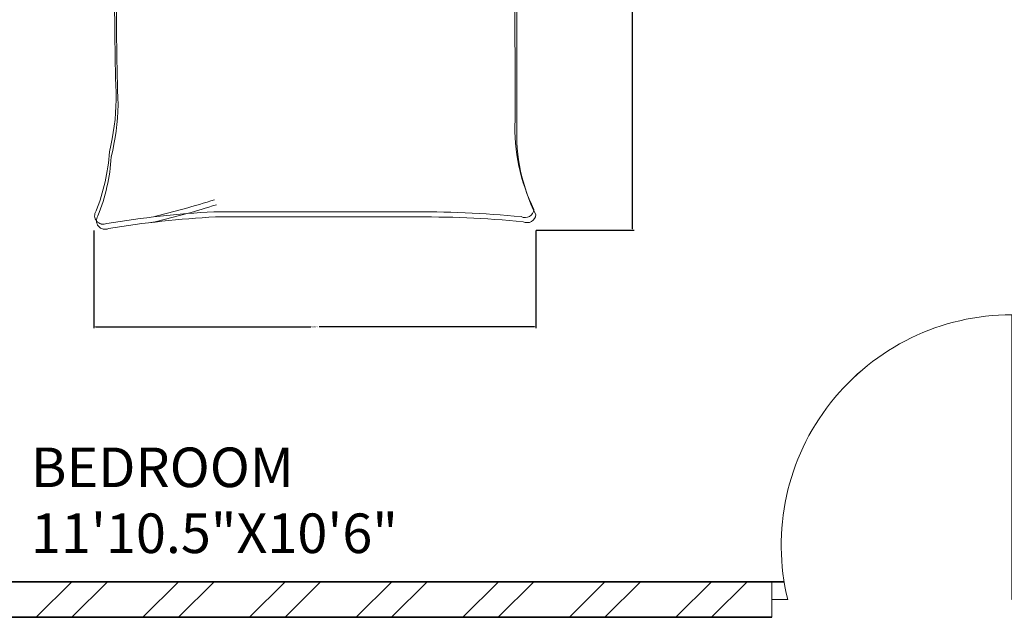
# Model space of a CAD drawing. Units: inches. Extents: x 2120 to 4013, y 1390 to 3019.
# Tile 40 of 59: x 2736 to 2861, y 2213 to 2289. Entities that reach past the tile are written whole.
import ezdxf

# ---------------------------------------------------------------- set-up
doc = ezdxf.new("R2010")
doc.units = ezdxf.units.IN
for name, color, linetype, lineweight in [('A-ANNO-DIMS', 2, 'Continuous', 18), ('A-AREA-IDEN', 7, 'Continuous', 18), ('A-DOOR', 3, 'Continuous', 18), ('A-FURN', 8, 'Continuous', 13), ('A-WALL', 7, 'Continuous', 35), ('A-WALL-PATT', 252, 'Continuous', 13)]:
    doc.layers.add(name, color=color, linetype=linetype, lineweight=lineweight)
doc.styles.get("Standard").update_dxf_attribs({"font": 'arial.ttf'})
doc.dimstyles.get("Standard").update_dxf_attribs({"dimtxt": 0.18, "dimasz": 0.18, "dimexe": 0.18, "dimexo": 0.0625, "dimgap": 0.09, "dimtad": 0, "dimtih": 1, "dimtoh": 1, "dimdec": 4, "dimzin": 0, "dimdsep": 46, "dimtxsty": 'Standard', "dimcen": 0.09, "dimadec": 0, "dimazin": 0, "dimtfac": 1, "dimtdec": 4, "dimtofl": 0, "dimtmove": 0, "dimatfit": 3, "dimfxl": 1, "dimtolj": 1, "dimtzin": 0, "dimarcsym": 0})

# ---------------------------------------------------------------- blocks, each defined once
blk = doc.blocks.new('BED-DOUBLE-PLAN')
for p, q in [((3.48, 63.34), (3.48, 81.45)), ((3.48, 81.45), (51.27, 81.45)), ((51.27, 81.45), (51.27, 54.84)), ((3.48, 79.91), (51.27, 79.91)), ((3.7, 62.7), (3.7, 80.81)), ((51.5, 80.81), (51.5, 54.2)), ((3.7, 79.27), (51.5, 79.27)), ((3.9, 78.11), (8.18, 78.44)), ((8.18, 78.44), (8.29, 78.42)), ((8.29, 78.42), (12.11, 78.13)), ((14.86, 77.7), (16.88, 78.42)), ((16.88, 78.42), (19.77, 79.14)), ((17.11, 77.78), (20, 78.5)), ((19.77, 79.14), (20.09, 79.14)), ((20, 78.5), (20.32, 78.5)), ((20.09, 79.14), (24.54, 79)), ((20.32, 78.5), (24.77, 78.36)), ((24.54, 79), (25.98, 79.58)), ((24.77, 78.36), (26.21, 78.94)), ((25.98, 79.58), (26.56, 74.23)), ((26.21, 78.94), (26.79, 73.59)), ((27.98, 78.95), (27.73, 73.58)), ((29.46, 78.47), (27.98, 78.95)), ((33.89, 78.89), (29.46, 78.47)), ((34.21, 78.91), (33.89, 78.89)), ((37.14, 78.37), (34.21, 78.91)), ((41.92, 78.38), (36.5, 77.02)), ((45.71, 78.9), (41.92, 78.38)), ((50.11, 78.89), (44.71, 78.99)), ((44.71, 78.99), (45.71, 78.9)), ((50.11, 78.89), (49.73, 75.68)), ((3.9, 78.13), (4.47, 74.95)), ((4.12, 77.49), (4.7, 74.31)), ((4.13, 77.47), (8.41, 77.8)), ((8.41, 77.8), (8.51, 77.78)), ((8.51, 77.78), (12.34, 77.49)), ((12.11, 78.13), (17.6, 77.12)), ((12.34, 77.49), (17.83, 76.48)), ((15.08, 77.06), (17.11, 77.78)), ((28.21, 78.32), (27.96, 72.94)), ((29.69, 77.83), (28.21, 78.32)), ((34.11, 78.25), (29.69, 77.83)), ((34.43, 78.27), (34.11, 78.25)), ((37.37, 77.73), (34.43, 78.27)), ((42.14, 77.74), (36.72, 76.38)), ((39.2, 77.77), (37.14, 78.37)), ((39.43, 77.13), (37.37, 77.73)), ((45.94, 78.26), (42.14, 77.74)), ((50.34, 78.25), (44.94, 78.35)), ((44.94, 78.35), (45.94, 78.26)), ((50.34, 78.25), (49.96, 75.04)), ((4.47, 74.95), (4.04, 72.35)), ((5.05, 72.49), (6.06, 75.24)), ((49.31, 73.19), (48.13, 75.87)), ((49.54, 72.55), (48.36, 75.23)), ((49.73, 75.68), (50.33, 73.11)), ((49.96, 75.04), (50.56, 72.47)), ((4.7, 74.31), (4.27, 71.71)), ((5.28, 71.85), (6.29, 74.6)), ((26.56, 74.23), (27.14, 71.05)), ((26.79, 73.59), (27.37, 70.41)), ((27.73, 73.58), (27.36, 70.37)), ((4.04, 72.35), (4.62, 71.33)), ((4.47, 68.88), (5.05, 72.49)), ((27.96, 72.94), (27.58, 69.73)), ((50.11, 69.62), (49.31, 73.19)), ((50.34, 68.98), (49.54, 72.55)), ((50.33, 73.11), (49.82, 72.06)), ((50.56, 72.47), (50.04, 71.42)), ((4.27, 71.71), (4.85, 70.7)), ((4.7, 68.24), (5.28, 71.85)), ((27.14, 71.05), (27.14, 69.74)), ((27.14, 69.74), (26.56, 67.86)), ((27.36, 70.37), (27.44, 69.07)), ((27.37, 70.41), (27.37, 69.1)), ((27.58, 69.73), (27.67, 68.43)), ((4.76, 67.29), (4.47, 68.88)), ((27.37, 69.1), (26.79, 67.23)), ((27.44, 69.07), (28.13, 67.23)), ((27.67, 68.43), (28.36, 66.59)), ((49.92, 68.01), (50.11, 69.62)), ((50.15, 67.37), (50.34, 68.98)), ((4.19, 64.11), (4.76, 67.29)), ((4.99, 66.65), (4.7, 68.24)), ((26.56, 67.86), (26.56, 65.18)), ((26.79, 67.23), (26.79, 64.54)), ((28.13, 67.23), (28.3, 64.55)), ((50.7, 64.87), (49.92, 68.01)), ((50.93, 64.23), (50.15, 67.37)), ((4.41, 63.47), (4.99, 66.65)), ((24.1, 65.18), (20.96, 66.27)), ((28.36, 66.59), (28.53, 63.91)), ((30.75, 64.71), (33.82, 65.99)), ((9.28, 64.83), (4.19, 64.11)), ((6.38, 65.82), (10.42, 65.15)), ((6.61, 65.18), (10.64, 64.51)), ((10.42, 65.15), (9.28, 64.83)), ((10.42, 65.15), (17.43, 64.72)), ((17.43, 64.72), (19.39, 65.28)), ((19.39, 65.28), (24.52, 64.87)), ((24.33, 64.54), (21.19, 65.63)), ((26.56, 65.18), (24.1, 65.18)), ((28.3, 64.55), (30.75, 64.71)), ((30.98, 64.07), (34.05, 65.35)), ((32.57, 65.82), (36.6, 65.15)), ((32.79, 65.18), (36.83, 64.51)), ((36.6, 65.15), (43.61, 64.72)), ((43.61, 64.72), (45.57, 65.28)), ((45.57, 65.28), (50.7, 64.87)), ((9.51, 64.19), (4.41, 63.47)), ((10.64, 64.51), (9.51, 64.19)), ((10.64, 64.51), (17.65, 64.08)), ((17.65, 64.08), (19.61, 64.64)), ((19.61, 64.64), (24.75, 64.23)), ((26.79, 64.54), (24.33, 64.54)), ((28.53, 63.91), (30.98, 64.07)), ((30.26, 64.06), (34.45, 57.57)), ((40.65, 61.13), (32.31, 64.06)), ((36.83, 64.51), (43.84, 64.08)), ((43.84, 64.08), (45.8, 64.64)), ((45.8, 64.64), (50.93, 64.23)), ((30.49, 63.42), (34.68, 56.93)), ((40.87, 60.49), (32.54, 63.42)), ((46.22, 59.12), (40.65, 61.13)), ((46.45, 58.48), (40.87, 60.49)), ((49.16, 56.95), (46.22, 59.12)), ((49.39, 56.31), (46.45, 58.48)), ((34.45, 57.57), (36.15, 53.08)), ((34.68, 56.93), (36.38, 52.44)), ((52.87, 53.7), (49.16, 56.95)), ((53.1, 53.06), (49.39, 56.31)), ((51.33, 53.08), (52.87, 53.7)), ((52.95, 51.96), (52.87, 53.7, 3.87)), ((36.15, 53.08), (36.46, 51.07)), ((36.38, 52.44), (36.69, 50.43)), ((38.94, 51.69), (40.96, 52.62)), ((40.96, 52.62), (44.36, 53.08)), ((41.18, 51.98), (44.59, 52.44)), ((44.36, 53.08), (48.23, 53.39)), ((44.59, 52.44), (48.46, 52.75)), ((48.23, 53.39), (51.33, 53.08)), ((48.46, 52.75), (51.56, 52.44)), ((51.56, 52.44), (53.1, 53.06)), ((53.18, 51.32), (53.1, 53.06, 3.87)), ((36.46, 51.07), (38.94, 51.69)), ((36.69, 50.43), (39.17, 51.05)), ((39.17, 51.05), (41.18, 51.98)), ((15.06, 2.2), (39.68, 2.2)), ((15.29, 1.56), (39.91, 1.56))]:
    blk.add_line(p, q)
for centre, radius, start, end in [((21.36, -100.61), 164.97, 86.0865, 96.7821), ((21.59, -101.25), 164.97, 86.0865, 96.7821), ((85.16, 61.35), 83.31, 178.7218, 185.604), ((85.39, 60.71), 83.31, 178.7218, 185.604), ((17.76, -74.87), 129.02, 81.7845, 96.9006), ((17.99, -75.51), 129.02, 81.7845, 96.9006), ((-167.31, 50.27), 170.11, 358.4762, 1.0082), ((-167.08, 49.63), 170.11, 358.4762, 1.0082), ((43.74, 46.38), 6.22, 78.6608, 113.7384), ((51.33, 88.1), 36.18, 259.8763, 272.5657), ((36.64, 51.01), 0.185, 160.2464, 271.1377), ((31.16, 79.96), 29.65, 280.6617, 289.8806), ((31.38, 79.32), 29.65, 280.6617, 289.8806), ((43.97, 45.74), 6.22, 78.6608, 113.7384), ((51.56, 87.46), 36.18, 259.8763, 272.5657), ((182.27, 45.13), 129.5, 176.9791, 183.8365), ((182.5, 44.49), 129.5, 176.9791, 183.8365), ((36.87, 50.37), 0.185, 160.2464, 271.1377), ((484.82, 30.83), 482.31, 178.2277, 181.7185), ((485.05, 30.19), 482.31, 178.2277, 181.7185), ((-4508.74, 13.62), 4561.86, 0.00217, 0.28689), ((-4508.51, 12.99), 4561.86, 0.00217, 0.28689), ((-26.9, 16.93), 29.63, 346.0648, 358.9113), ((-26.67, 16.29), 29.63, 346.0648, 358.9113), ((76.16, 12.78), 23.07, 177.4714, 206.4681), ((76.39, 12.14), 23.07, 177.4714, 206.4681), ((-21.66, 11.17), 23.56, 337.9751, 356.652), ((-21.43, 10.53), 23.56, 337.9751, 356.652), ((-17.22, 105.16), 106.46, 283.3832, 287.7053), ((-16.99, 104.52), 106.46, 283.3832, 287.7053), ((54.41, 2.58), 1.1, 242.6588, 356.02), ((1.09, 1.73), 1.09, 146.1736, 293.4781), ((1.32, 1.09), 1.09, 146.1736, 293.4781), ((21.43, -119.39), 121.76, 92.9958, 99.4091), ((21.66, -120.03), 121.76, 92.9958, 99.4091), ((41.15, -130.83), 133.04, 84.4998, 90.6351), ((41.38, -131.47), 133.04, 84.4998, 90.6351), ((54.64, 1.94), 1.1, 242.6588, 356.02)]:
    blk.add_arc(centre, radius, start, end)
blk = doc.blocks.new('DOOR-SWING-36IN-103p63DEG')
for p, q in [((30.32, 2.25), (30.32, 38.25)), ((0, 4.5), (0, 0)), ((32.32, 4.5), (32.32, 0)), ((0, 0), (0, 2.25)), ((0, 2.25), (2, 2.25)), ((32.32, 2.25), (30.32, 2.25)), ((32.32, 0), (32.32, 2.25))]:
    blk.add_line(p, q)
blk.add_arc((30.32, 9.11), 29.14, 90, 193.6269)
blk = doc.blocks.new('*D73')
at = {"layer": 'A-ANNO-DIMS', "color": 0, "lineweight": -2, "transparency": 16777216}
for p, q in [((2801.55, 2343.53), (2813.9, 2343.53)), ((2813.72, 2343.35), (2813.72, 2302.94)), ((2813.72, 2262.16), (2813.72, 2302.57)), ((2801.55, 2261.98), (2813.9, 2261.98))]:
    blk.add_line(p, q, dxfattribs=at)
at = {"layer": 'A-ANNO-DIMS', "color": 0, "transparency": 16777216}
for points in [[(2813.69, 2343.35), (2813.75, 2343.35), (2813.72, 2343.53)], [(2813.69, 2262.16), (2813.75, 2262.16), (2813.72, 2261.98)]]:
    blk.add_solid(points, dxfattribs=at)
at = {"layer": 'Defpoints', "color": 0, "transparency": 16777216}
for p in [(2801.49, 2343.53), (2813.72, 2343.53), (2801.49, 2261.98)]:
    blk.add_point(p, dxfattribs=at)
at = {"layer": 'A-ANNO-DIMS', "color": 0, "transparency": 16777216, "insert": (2813.72, 2302.76), "char_height": 0.18, "attachment_point": 5}
blk.add_mtext('\\A1;BED 82 TYP.', dxfattribs=at)
blk = doc.blocks.new('*D74')
at = {"layer": 'A-ANNO-DIMS', "color": 0, "lineweight": -2, "transparency": 16777216}
for p, q in [((2745.67, 2261.92), (2745.67, 2249.57)), ((2801.49, 2261.92), (2801.49, 2249.57)), ((2745.85, 2249.75), (2773.05, 2249.75)), ((2801.31, 2249.75), (2774.11, 2249.75))]:
    blk.add_line(p, q, dxfattribs=at)
at = {"layer": 'A-ANNO-DIMS', "color": 0, "transparency": 16777216}
for points in [[(2745.85, 2249.78), (2745.85, 2249.72), (2745.67, 2249.75)], [(2801.31, 2249.78), (2801.31, 2249.72), (2801.49, 2249.75)]]:
    blk.add_solid(points, dxfattribs=at)
at = {"layer": 'Defpoints', "color": 0, "transparency": 16777216}
for p in [(2745.67, 2261.98), (2801.49, 2261.98), (2801.49, 2249.75)]:
    blk.add_point(p, dxfattribs=at)
at = {"layer": 'A-ANNO-DIMS', "color": 0, "transparency": 16777216, "insert": (2773.58, 2249.75), "char_height": 0.18, "attachment_point": 5}
blk.add_mtext('\\A1;56 TYP.', dxfattribs=at)

msp = doc.modelspace()

# ---------------------------------------------------------------- hatches: boundary and pattern name
at = {"layer": 'A-WALL-PATT'}
h = msp.add_hatch(dxfattribs=at)
h.set_pattern_fill('ANSI32', color=256)
h.paths.add_polyline_path([(2271.7331, 2343.531), (2283.3788, 2343.531), (2283.3788, 2348.031), (2283.3788, 2352.5306), (2262.7331, 2352.5306), (2262.7331, 2182.638), (2267.2331, 2182.638), (2271.7331, 2182.638), (2271.7331, 2219.031), (2391.7331, 2219.031), (2391.7331, 2214.189), (2393.9831, 2214.189), (2396.2331, 2214.189), (2396.2331, 2219.031), (2420.2331, 2219.031), (2420.2331, 2225.7535), (2417.2197, 2225.7535), (2415.7331, 2225.7535), (2415.7331, 2223.5306), (2271.7331, 2223.5306)])
h.paths.add_polyline_path([(2380.0942, 2352.5306), (2343.3788, 2352.5306), (2343.3788, 2343.531), (2363.2331, 2343.531), (2363.2331, 2288.8489), (2365.4831, 2288.8489), (2367.7331, 2288.8489), (2367.7331, 2343.531), (2380.0942, 2343.531)], flags=17)
h.paths.add_polyline_path([(2432.4339, 2352.5306), (2404.0943, 2352.5306), (2404.0943, 2343.531), (2415.7331, 2343.531), (2415.7331, 2264.0306), (2367.7331, 2264.0306), (2367.7331, 2266.4872), (2363.2331, 2266.4872), (2363.2331, 2259.531), (2367.7331, 2259.531), (2415.7331, 2259.531), (2415.7331, 2255.0658), (2420.2331, 2255.0658), (2420.2331, 2259.531), (2424.5717, 2259.531), (2424.5717, 2261.781), (2424.5717, 2264.0306), (2420.2331, 2264.0306), (2420.2331, 2343.531), (2432.4339, 2343.531)])
h.paths.add_polyline_path([(2508.9115, 2352.5306), (2456.4339, 2352.5306), (2456.4339, 2343.531), (2468.2331, 2343.531), (2468.2331, 2264.0306), (2448.0487, 2264.0306), (2448.0487, 2259.531), (2468.2331, 2259.531), (2468.2331, 2255.5496), (2472.7331, 2255.5496), (2472.7331, 2343.531), (2508.9115, 2343.531)])
h.paths.add_polyline_path([(2637.7331, 2352.5306), (2544.9116, 2352.5306), (2544.9116, 2343.531), (2589.7331, 2343.531), (2633.2331, 2343.531), (2637.7331, 2343.531)])
h.paths.add_polyline_path([(2594.2331, 2343.5306), (2589.7331, 2343.5306), (2589.7331, 2259.5306), (2589.7331, 2252.4915), (2591.9831, 2252.4915), (2594.2331, 2252.4915)])
h.paths.add_polyline_path([(2637.7331, 2223.5306), (2594.2331, 2223.5306), (2594.2331, 2230.1988), (2591.9831, 2230.1988), (2589.7331, 2230.1988), (2589.7331, 2223.5306), (2472.7331, 2223.5306), (2468.2331, 2223.5306), (2468.2331, 2219.031), (2628.7331, 2219.031), (2628.7331, 2138.031), (2637.7331, 2138.031)])
h.paths.add_polyline_path([(3822.6535, 2458.4402), (3874.9468, 2458.4402), (3874.9468, 2476.9866), (3822.6535, 2476.9866)], flags=9)
h.paths.add_polyline_path([(3834.6921, 2781.8174), (3935.9206, 2781.8174), (3935.9206, 2800.3638), (3834.6921, 2800.3638)], flags=9)
h.paths.add_polyline_path([(3832.2843, 2837.9683), (3884.5776, 2837.9683), (3884.5776, 2856.5146), (3832.2843, 2856.5146)], flags=9)
h.paths.add_polyline_path([(3830.9388, 2861.4782), (3956.8958, 2861.4782), (3956.8958, 2880.0245), (3830.9388, 2880.0245)], flags=9)
h.paths.add_polyline_path([(3870.6966, 2352.5752), (3887.9272, 2352.5752), (3887.9272, 2377.3037), (3870.6966, 2377.3037)], flags=9)
h.paths.add_polyline_path([(3289.2701, 2413.161), (3435.2223, 2413.161), (3435.2223, 2450.2538), (3289.2701, 2450.2538)], flags=9)
h.paths.add_polyline_path([(2487.6944, 2414.3601), (2637.8335, 2414.3601), (2637.8335, 2451.4528), (2487.6944, 2451.4528)], flags=9)
h.paths.add_polyline_path([(2567.3724, 1457.9199), (2815.296, 1457.9199), (2815.296, 1495.0127), (2567.3724, 1495.0127)], flags=9)
h.paths.add_polyline_path([(2655.3825, 2093.2363), (2685.9555, 2093.2363), (2685.9555, 2111.8937), (2655.3825, 2111.8937)], flags=9)
h.paths.add_polyline_path([(2543.9218, 1550.6671), (2587.8406, 1550.6671), (2587.8406, 1569.3244), (2543.9218, 1569.3244)], flags=9)
h.paths.add_polyline_path([(2905.1384, 1543.8113), (2949.0572, 1543.8113), (2949.0572, 1562.4686), (2905.1384, 1562.4686)], flags=9)
h.paths.add_polyline_path([(2736.4118, 1702.4736), (2784.2153, 1702.4736), (2784.2153, 1721.1309), (2736.4118, 1721.1309)], flags=9)
h.paths.add_polyline_path([(2912.8666, 1710.4168), (2951.707, 1710.4168), (2951.707, 1729.0741), (2912.8666, 1729.0741)], flags=9)
h.paths.add_polyline_path([(2923.5785, 1763.5038), (2959.7279, 1763.5038), (2959.7279, 1782.1611), (2923.5785, 1782.1611)], flags=9)
h.paths.add_polyline_path([(2925.2114, 1809.6137), (2967.1861, 1809.6137), (2967.1861, 1828.271), (2925.2114, 1828.271)], flags=9)
h.paths.add_polyline_path([(2996.2711, 1878.9003), (2996.2711, 1913.109), (2977.6138, 1913.109), (2977.6138, 1878.9003)], flags=9)
h.paths.add_polyline_path([(2883.0859, 1895.7192), (2927.1855, 1895.7192), (2927.1855, 1914.3766), (2883.0859, 1914.3766)], flags=9)
h.paths.add_polyline_path([(2787.3924, 1810.8013), (2841.0213, 1810.8013), (2841.0213, 1829.4587), (2787.3924, 1829.4587)], flags=9)
h.paths.add_polyline_path([(2775.6399, 2101.7395), (2829.2689, 2101.7395), (2829.2689, 2120.3968), (2775.6399, 2120.3968)], flags=9)
h.paths.add_polyline_path([(2913.0263, 2075.817), (2951.8667, 2075.817), (2951.8667, 2094.4744), (2913.0263, 2094.4744)], flags=9)
h.paths.add_polyline_path([(2929.966, 2133.3669), (2966.1154, 2133.3669), (2966.1154, 2152.0243), (2929.966, 2152.0243)], flags=9)
h.paths.add_polyline_path([(2932.7502, 2182.6088), (2968.8996, 2182.6088), (2968.8996, 2201.2662), (2932.7502, 2201.2662)], flags=9)
h.paths.add_polyline_path([(2996.0681, 2266.3173), (2996.0681, 2300.5261), (2977.4108, 2300.5261), (2977.4108, 2266.3173)], flags=9)
h.paths.add_polyline_path([(2885.1039, 2279.2186), (2929.2035, 2279.2186), (2929.2035, 2297.8759), (2885.1039, 2297.8759)], flags=9)
h.paths.add_polyline_path([(2735.7042, 2218.3197), (2783.5078, 2218.3197), (2783.5078, 2236.9771), (2735.7042, 2236.9771)], flags=9)
h.paths.add_polyline_path([(2635.6049, 2044.0085), (2648.9678, 2044.0085), (2648.9678, 2054.312), (2635.6049, 2054.312)], flags=9)
h.paths.add_polyline_path([(2714.0148, 1923.0473), (2727.3777, 1923.0473), (2727.3777, 1933.3508), (2714.0148, 1933.3508)], flags=9)
h.paths.add_polyline_path([(2709.0345, 1988.1628), (2722.3974, 1988.1628), (2722.3974, 1998.4663), (2709.0345, 1998.4663)], flags=9)
h.paths.add_polyline_path([(2592.8935, 1962.1763), (2606.2564, 1962.1763), (2606.2564, 1972.4799), (2592.8935, 1972.4799)], flags=9)
h.paths.add_polyline_path([(2618.3996, 1985.9724), (2644.1942, 1985.9724), (2644.1942, 1996.2759), (2618.3996, 1996.2759)], flags=9)
h.paths.add_polyline_path([(2601.279, 1920.5869), (2614.6419, 1920.5869), (2614.6419, 1930.8904), (2601.279, 1930.8904)], flags=9)
h.paths.add_polyline_path([(2692.3278, 1932.7645), (2704.5311, 1932.7645), (2704.5311, 1943.0681), (2692.3278, 1943.0681)], flags=9)
h.paths.add_polyline_path([(2311.122, 1672.7318), (2355.0408, 1672.7318), (2355.0408, 1691.3892), (2311.122, 1691.3892)], flags=9)
h.paths.add_polyline_path([(2456.2551, 1632.3198), (2492.4796, 1632.3198), (2492.4796, 1650.9772), (2456.2551, 1650.9772)], flags=9)
h.paths.add_polyline_path([(2401.0766, 1631.4793), (2437.301, 1631.4793), (2437.301, 1650.1367), (2401.0766, 1650.1367)], flags=9)
h.paths.add_polyline_path([(2546.7054, 1700.9235), (2594.509, 1700.9235), (2594.509, 1719.5809), (2546.7054, 1719.5809)], flags=9)
h.paths.add_polyline_path([(2445.4866, 1766.9937), (2497.5261, 1766.9937), (2497.5261, 1785.651), (2445.4866, 1785.651)], flags=9)
h.paths.add_polyline_path([(2287.9992, 1739.7675), (2326.8396, 1739.7675), (2326.8396, 1758.4248), (2287.9992, 1758.4248)], flags=9)
h.paths.add_polyline_path([(2458.5279, 1924.7607), (2510.5675, 1924.7607), (2510.5675, 1943.4181), (2458.5279, 1943.4181)], flags=9)
h.paths.add_polyline_path([(2309.2811, 1902.7642), (2345.4305, 1902.7642), (2345.4305, 1921.4215), (2309.2811, 1921.4215)], flags=9)
h.paths.add_polyline_path([(2490.7554, 2018.9392), (2530.7896, 2018.9392), (2530.7896, 2037.5965), (2490.7554, 2037.5965)], flags=9)
h.paths.add_polyline_path([(2402.143, 2024.7393), (2438.5414, 2024.7393), (2438.5414, 2043.3966), (2402.143, 2043.3966)], flags=9)
h.paths.add_polyline_path([(2287.856, 1931.7926), (2326.6964, 1931.7926), (2326.6964, 1950.4499), (2287.856, 1950.4499)], flags=9)
h.paths.add_polyline_path([(2281.7979, 2193.5771), (2320.6383, 2193.5771), (2320.6383, 2212.2344), (2281.7979, 2212.2344)], flags=25)
h.paths.add_polyline_path([(2484.0754, 2093.892), (2536.115, 2093.892), (2536.115, 2112.5494), (2484.0754, 2112.5494)], flags=9)
h.paths.add_polyline_path([(2624.7948, 2281.8639), (2624.7948, 2311.4137), (2606.1375, 2311.4137), (2606.1375, 2281.8639)], flags=9)
h.paths.add_polyline_path([(2507.5036, 2290.3639), (2541.934, 2290.3639), (2541.934, 2309.0212), (2507.5036, 2309.0212)], flags=9)
h.paths.add_polyline_path([(2423.1076, 2285.2202), (2459.332, 2285.2202), (2459.332, 2303.8776), (2423.1076, 2303.8776)], flags=9)
h.paths.add_polyline_path([(2374.5467, 2289.6272), (2410.7711, 2289.6272), (2410.7711, 2308.2846), (2374.5467, 2308.2846)], flags=25)
h.paths.add_polyline_path([(2277.4907, 2227.5651), (2316.3311, 2227.5651), (2316.3311, 2246.2224), (2277.4907, 2246.2224)], flags=25)
h.paths.add_polyline_path([(2655.3825, 2093.2367), (2685.9555, 2093.2367), (2685.9555, 2111.894), (2655.3825, 2111.894)], flags=9)
h.paths.add_polyline_path([(2543.9217, 1550.6674), (2587.8406, 1550.6674), (2587.8406, 1569.3247), (2543.9217, 1569.3247)], flags=9)
h.paths.add_polyline_path([(2905.1384, 1543.8116), (2949.0572, 1543.8116), (2949.0572, 1562.4689), (2905.1384, 1562.4689)], flags=9)
h.paths.add_polyline_path([(2736.4118, 1702.4739), (2784.2153, 1702.4739), (2784.2153, 1721.1312), (2736.4118, 1721.1312)], flags=9)
h.paths.add_polyline_path([(2912.8666, 1710.4171), (2951.707, 1710.4171), (2951.707, 1729.0744), (2912.8666, 1729.0744)], flags=9)
h.paths.add_polyline_path([(2923.5785, 1763.5041), (2959.7279, 1763.5041), (2959.7279, 1782.1614), (2923.5785, 1782.1614)], flags=9)
h.paths.add_polyline_path([(2925.2114, 1809.614), (2967.1861, 1809.614), (2967.1861, 1828.2713), (2925.2114, 1828.2713)], flags=9)
h.paths.add_polyline_path([(2996.2711, 1878.9006), (2996.2711, 1913.1094), (2977.6137, 1913.1094), (2977.6137, 1878.9006)], flags=9)
h.paths.add_polyline_path([(2883.0859, 1895.7195), (2927.1855, 1895.7195), (2927.1855, 1914.3769), (2883.0859, 1914.3769)], flags=9)
h.paths.add_polyline_path([(2787.3924, 1810.8016), (2841.0213, 1810.8016), (2841.0213, 1829.459), (2787.3924, 1829.459)], flags=9)
h.paths.add_polyline_path([(2775.6399, 2101.7398), (2829.2688, 2101.7398), (2829.2688, 2120.3971), (2775.6399, 2120.3971)], flags=9)
h.paths.add_polyline_path([(2913.0263, 2075.8173), (2951.8667, 2075.8173), (2951.8667, 2094.4747), (2913.0263, 2094.4747)], flags=9)
h.paths.add_polyline_path([(2929.966, 2133.3672), (2966.1154, 2133.3672), (2966.1154, 2152.0246), (2929.966, 2152.0246)], flags=9)
h.paths.add_polyline_path([(2932.7502, 2182.6091), (2968.8996, 2182.6091), (2968.8996, 2201.2665), (2932.7502, 2201.2665)], flags=9)
h.paths.add_polyline_path([(2996.0681, 2266.3176), (2996.0681, 2300.5264), (2977.4108, 2300.5264), (2977.4108, 2266.3176)], flags=9)
h.paths.add_polyline_path([(2885.1039, 2279.2189), (2929.2035, 2279.2189), (2929.2035, 2297.8762), (2885.1039, 2297.8762)], flags=9)
h.paths.add_polyline_path([(2735.7042, 2218.32), (2783.5078, 2218.32), (2783.5078, 2236.9774), (2735.7042, 2236.9774)], flags=9)
h.paths.add_polyline_path([(2635.6048, 2044.0088), (2648.9677, 2044.0088), (2648.9677, 2054.3123), (2635.6048, 2054.3123)], flags=9)
h.paths.add_polyline_path([(2714.0148, 1923.0476), (2727.3777, 1923.0476), (2727.3777, 1933.3511), (2714.0148, 1933.3511)], flags=9)
h.paths.add_polyline_path([(2709.0345, 1988.1631), (2722.3974, 1988.1631), (2722.3974, 1998.4666), (2709.0345, 1998.4666)], flags=9)
h.paths.add_polyline_path([(2592.8935, 1962.1766), (2606.2564, 1962.1766), (2606.2564, 1972.4802), (2592.8935, 1972.4802)], flags=9)
h.paths.add_polyline_path([(2618.3995, 1985.9727), (2644.1942, 1985.9727), (2644.1942, 1996.2762), (2618.3995, 1996.2762)], flags=9)
h.paths.add_polyline_path([(2601.279, 1920.5872), (2614.6419, 1920.5872), (2614.6419, 1930.8908), (2601.279, 1930.8908)], flags=9)
h.paths.add_polyline_path([(2692.3278, 1932.7648), (2704.5311, 1932.7648), (2704.5311, 1943.0684), (2692.3278, 1943.0684)], flags=9)
h.paths.add_polyline_path([(2311.122, 1672.7321), (2355.0408, 1672.7321), (2355.0408, 1691.3895), (2311.122, 1691.3895)], flags=9)
h.paths.add_polyline_path([(2456.2551, 1632.3201), (2492.4795, 1632.3201), (2492.4795, 1650.9775), (2456.2551, 1650.9775)], flags=9)
h.paths.add_polyline_path([(2401.0766, 1631.4796), (2437.301, 1631.4796), (2437.301, 1650.137), (2401.0766, 1650.137)], flags=9)
h.paths.add_polyline_path([(2546.7054, 1700.9238), (2594.509, 1700.9238), (2594.509, 1719.5812), (2546.7054, 1719.5812)], flags=9)
h.paths.add_polyline_path([(2445.4866, 1766.994), (2497.5261, 1766.994), (2497.5261, 1785.6513), (2445.4866, 1785.6513)], flags=9)
h.paths.add_polyline_path([(2287.9992, 1739.7678), (2326.8396, 1739.7678), (2326.8396, 1758.4251), (2287.9992, 1758.4251)], flags=9)
h.paths.add_polyline_path([(2458.5279, 1924.7611), (2510.5675, 1924.7611), (2510.5675, 1943.4184), (2458.5279, 1943.4184)], flags=9)
h.paths.add_polyline_path([(2309.2811, 1902.7645), (2345.4305, 1902.7645), (2345.4305, 1921.4218), (2309.2811, 1921.4218)], flags=9)
h.paths.add_polyline_path([(2490.7554, 2018.9395), (2530.7895, 2018.9395), (2530.7895, 2037.5968), (2490.7554, 2037.5968)], flags=9)
h.paths.add_polyline_path([(2402.143, 2024.7396), (2438.5413, 2024.7396), (2438.5413, 2043.3969), (2402.143, 2043.3969)], flags=9)
h.paths.add_polyline_path([(2287.856, 1931.7929), (2326.6964, 1931.7929), (2326.6964, 1950.4502), (2287.856, 1950.4502)], flags=9)
h.paths.add_polyline_path([(2281.7979, 2193.5774), (2320.6383, 2193.5774), (2320.6383, 2212.2347), (2281.7979, 2212.2347)], flags=25)
h.paths.add_polyline_path([(2484.0754, 2093.8924), (2536.115, 2093.8924), (2536.115, 2112.5497), (2484.0754, 2112.5497)], flags=9)
h.paths.add_polyline_path([(2624.7948, 2281.8642), (2624.7948, 2311.414), (2606.1374, 2311.414), (2606.1374, 2281.8642)], flags=9)
h.paths.add_polyline_path([(2507.5035, 2290.3642), (2541.934, 2290.3642), (2541.934, 2309.0215), (2507.5035, 2309.0215)], flags=9)
h.paths.add_polyline_path([(2423.1075, 2285.2205), (2459.332, 2285.2205), (2459.332, 2303.8779), (2423.1075, 2303.8779)], flags=9)
h.paths.add_polyline_path([(2374.5467, 2289.6275), (2410.7711, 2289.6275), (2410.7711, 2308.2849), (2374.5467, 2308.2849)], flags=25)
h.paths.add_polyline_path([(2277.4907, 2227.5654), (2316.3311, 2227.5654), (2316.3311, 2246.2227), (2277.4907, 2246.2227)], flags=25)
h = msp.add_hatch(dxfattribs=at)
h.set_pattern_fill('ANSI32', color=256)
h.paths.add_polyline_path([(2271.7331, 1980.389), (2262.7331, 1980.389), (2262.7331, 1912.8434), (2267.2331, 1912.8434), (2271.7331, 1912.8434), (2271.7331, 1922.531), (2351.2331, 1922.531), (2351.2331, 1901.4728), (2355.7331, 1901.4728), (2355.7331, 1922.531), (2357.9815, 1922.531), (2357.9815, 1926.5306), (2271.7331, 1926.5306)])
h.paths.add_polyline_path([(2589.2331, 1949.1622), (2584.7331, 1949.1622), (2580.2331, 1949.1622), (2580.2331, 1874.5306), (2355.7331, 1874.5306), (2355.7331, 1880.1922), (2351.2331, 1880.1922), (2351.2331, 1874.5306), (2271.7331, 1874.5306), (2271.7331, 1888.8431), (2262.7331, 1888.8431), (2262.7331, 1842.2909), (2267.2331, 1842.2909), (2271.7331, 1842.2909), (2271.7331, 1865.531), (2415.7331, 1865.531), (2415.7331, 1779.7286), (2420.2331, 1779.7286), (2420.2331, 1865.531), (2589.2331, 1865.531)])
h.paths.add_polyline_path([(2271.7331, 1782.2906), (2262.7331, 1782.2906), (2262.7331, 1711.4639), (2267.2331, 1711.4639), (2271.7331, 1711.4639), (2271.7331, 1738.031), (2420.2331, 1738.031), (2420.2331, 1742.531), (2420.2331, 1747.3376), (2417.9831, 1747.3376), (2415.7331, 1747.3376), (2415.7331, 1742.5306), (2271.7331, 1742.5306)])
h.paths.add_polyline_path([(2271.7331, 1627.031), (2362.3957, 1627.031), (2362.3957, 1629.281), (2362.3957, 1631.5306), (2271.7331, 1631.5306), (2271.7331, 1675.4636), (2262.7331, 1675.4636), (2262.7331, 1581.531), (2405.3032, 1581.531), (2405.3032, 1586.031), (2405.3032, 1590.5306), (2396.2331, 1590.5306), (2396.2331, 1691.4513), (2418.7206, 1691.4513), (2418.7206, 1695.951), (2396.2331, 1695.951), (2391.7331, 1695.951), (2391.7331, 1631.5306), (2386.7425, 1631.5306), (2386.7425, 1629.2806), (2386.7425, 1627.031), (2391.7331, 1627.031), (2391.7331, 1586.1709), (2271.7331, 1586.1709)])
h.paths.add_polyline_path([(2459.6703, 1590.5306), (2429.3032, 1590.5306), (2429.3032, 1581.531), (2459.6703, 1581.531), (2459.6703, 1586.031)])
h.paths.add_polyline_path([(2501.2331, 1590.531), (2501.2331, 1665.0195), (2498.9831, 1665.0195), (2496.7331, 1665.0195), (2496.7331, 1590.5306), (2483.8201, 1590.5306), (2483.8201, 1590.1579), (2483.6704, 1590.1579), (2483.6704, 1581.531), (2505.0196, 1581.531), (2505.0196, 1583.781), (2505.0196, 1586.0306), (2501.2331, 1586.0306)])
h.paths.add_polyline_path([(2544.1361, 1583.781), (2544.1361, 1586.0306), (2527.1368, 1586.0306), (2527.1368, 1583.7806), (2527.1368, 1581.531), (2544.1361, 1581.531)])
h.paths.add_polyline_path([(3822.6535, 2458.4402), (3874.9468, 2458.4402), (3874.9468, 2476.9866), (3822.6535, 2476.9866)], flags=9)
h.paths.add_polyline_path([(3834.6921, 2781.8174), (3935.9206, 2781.8174), (3935.9206, 2800.3638), (3834.6921, 2800.3638)], flags=9)
h.paths.add_polyline_path([(3832.2843, 2837.9683), (3884.5776, 2837.9683), (3884.5776, 2856.5146), (3832.2843, 2856.5146)], flags=9)
h.paths.add_polyline_path([(3830.9388, 2861.4782), (3956.8958, 2861.4782), (3956.8958, 2880.0245), (3830.9388, 2880.0245)], flags=9)
h.paths.add_polyline_path([(3870.6966, 2352.5752), (3887.9272, 2352.5752), (3887.9272, 2377.3037), (3870.6966, 2377.3037)], flags=9)
h.paths.add_polyline_path([(3289.2701, 2413.161), (3435.2223, 2413.161), (3435.2223, 2450.2538), (3289.2701, 2450.2538)], flags=9)
h.paths.add_polyline_path([(2487.6944, 2414.3601), (2637.8335, 2414.3601), (2637.8335, 2451.4528), (2487.6944, 2451.4528)], flags=9)
h.paths.add_polyline_path([(2567.3724, 1457.9199), (2815.296, 1457.9199), (2815.296, 1495.0127), (2567.3724, 1495.0127)], flags=9)
h.paths.add_polyline_path([(2655.3825, 2093.2363), (2685.9555, 2093.2363), (2685.9555, 2111.8937), (2655.3825, 2111.8937)], flags=9)
h.paths.add_polyline_path([(2543.9218, 1550.6671), (2587.8406, 1550.6671), (2587.8406, 1569.3244), (2543.9218, 1569.3244)], flags=9)
h.paths.add_polyline_path([(2905.1384, 1543.8113), (2949.0572, 1543.8113), (2949.0572, 1562.4686), (2905.1384, 1562.4686)], flags=9)
h.paths.add_polyline_path([(2736.4118, 1702.4736), (2784.2153, 1702.4736), (2784.2153, 1721.1309), (2736.4118, 1721.1309)], flags=9)
h.paths.add_polyline_path([(2912.8666, 1710.4168), (2951.707, 1710.4168), (2951.707, 1729.0741), (2912.8666, 1729.0741)], flags=9)
h.paths.add_polyline_path([(2923.5785, 1763.5038), (2959.7279, 1763.5038), (2959.7279, 1782.1611), (2923.5785, 1782.1611)], flags=9)
h.paths.add_polyline_path([(2925.2114, 1809.6137), (2967.1861, 1809.6137), (2967.1861, 1828.271), (2925.2114, 1828.271)], flags=9)
h.paths.add_polyline_path([(2996.2711, 1878.9003), (2996.2711, 1913.109), (2977.6138, 1913.109), (2977.6138, 1878.9003)], flags=9)
h.paths.add_polyline_path([(2883.0859, 1895.7192), (2927.1855, 1895.7192), (2927.1855, 1914.3766), (2883.0859, 1914.3766)], flags=9)
h.paths.add_polyline_path([(2787.3924, 1810.8013), (2841.0213, 1810.8013), (2841.0213, 1829.4587), (2787.3924, 1829.4587)], flags=9)
h.paths.add_polyline_path([(2775.6399, 2101.7395), (2829.2689, 2101.7395), (2829.2689, 2120.3968), (2775.6399, 2120.3968)], flags=9)
h.paths.add_polyline_path([(2913.0263, 2075.817), (2951.8667, 2075.817), (2951.8667, 2094.4744), (2913.0263, 2094.4744)], flags=9)
h.paths.add_polyline_path([(2929.966, 2133.3669), (2966.1154, 2133.3669), (2966.1154, 2152.0243), (2929.966, 2152.0243)], flags=9)
h.paths.add_polyline_path([(2932.7502, 2182.6088), (2968.8996, 2182.6088), (2968.8996, 2201.2662), (2932.7502, 2201.2662)], flags=9)
h.paths.add_polyline_path([(2996.0681, 2266.3173), (2996.0681, 2300.5261), (2977.4108, 2300.5261), (2977.4108, 2266.3173)], flags=9)
h.paths.add_polyline_path([(2885.1039, 2279.2186), (2929.2035, 2279.2186), (2929.2035, 2297.8759), (2885.1039, 2297.8759)], flags=9)
h.paths.add_polyline_path([(2735.7042, 2218.3197), (2783.5078, 2218.3197), (2783.5078, 2236.9771), (2735.7042, 2236.9771)], flags=9)
h.paths.add_polyline_path([(2635.6049, 2044.0085), (2648.9678, 2044.0085), (2648.9678, 2054.312), (2635.6049, 2054.312)], flags=9)
h.paths.add_polyline_path([(2714.0148, 1923.0473), (2727.3777, 1923.0473), (2727.3777, 1933.3508), (2714.0148, 1933.3508)], flags=9)
h.paths.add_polyline_path([(2709.0345, 1988.1628), (2722.3974, 1988.1628), (2722.3974, 1998.4663), (2709.0345, 1998.4663)], flags=9)
h.paths.add_polyline_path([(2592.8935, 1962.1763), (2606.2564, 1962.1763), (2606.2564, 1972.4799), (2592.8935, 1972.4799)], flags=9)
h.paths.add_polyline_path([(2618.3996, 1985.9724), (2644.1942, 1985.9724), (2644.1942, 1996.2759), (2618.3996, 1996.2759)], flags=9)
h.paths.add_polyline_path([(2601.279, 1920.5869), (2614.6419, 1920.5869), (2614.6419, 1930.8904), (2601.279, 1930.8904)], flags=9)
h.paths.add_polyline_path([(2692.3278, 1932.7645), (2704.5311, 1932.7645), (2704.5311, 1943.0681), (2692.3278, 1943.0681)], flags=9)
h.paths.add_polyline_path([(2311.122, 1672.7318), (2355.0408, 1672.7318), (2355.0408, 1691.3892), (2311.122, 1691.3892)], flags=25)
h.paths.add_polyline_path([(2456.2551, 1632.3198), (2492.4796, 1632.3198), (2492.4796, 1650.9772), (2456.2551, 1650.9772)], flags=9)
h.paths.add_polyline_path([(2401.0766, 1631.4793), (2437.301, 1631.4793), (2437.301, 1650.1367), (2401.0766, 1650.1367)], flags=9)
h.paths.add_polyline_path([(2546.7054, 1700.9235), (2594.509, 1700.9235), (2594.509, 1719.5809), (2546.7054, 1719.5809)], flags=9)
h.paths.add_polyline_path([(2445.4866, 1766.9937), (2497.5261, 1766.9937), (2497.5261, 1785.651), (2445.4866, 1785.651)], flags=9)
h.paths.add_polyline_path([(2287.9992, 1739.7675), (2326.8396, 1739.7675), (2326.8396, 1758.4248), (2287.9992, 1758.4248)], flags=24)
h.paths.add_polyline_path([(2458.5279, 1924.7607), (2510.5675, 1924.7607), (2510.5675, 1943.4181), (2458.5279, 1943.4181)], flags=25)
h.paths.add_polyline_path([(2309.2811, 1902.7642), (2345.4305, 1902.7642), (2345.4305, 1921.4215), (2309.2811, 1921.4215)], flags=25)
h.paths.add_polyline_path([(2490.7554, 2018.9392), (2530.7896, 2018.9392), (2530.7896, 2037.5965), (2490.7554, 2037.5965)], flags=9)
h.paths.add_polyline_path([(2402.143, 2024.7393), (2438.5414, 2024.7393), (2438.5414, 2043.3966), (2402.143, 2043.3966)], flags=9)
h.paths.add_polyline_path([(2287.856, 1931.7926), (2326.6964, 1931.7926), (2326.6964, 1950.4499), (2287.856, 1950.4499)], flags=25)
h.paths.add_polyline_path([(2281.7979, 2193.5771), (2320.6383, 2193.5771), (2320.6383, 2212.2344), (2281.7979, 2212.2344)], flags=9)
h.paths.add_polyline_path([(2484.0754, 2093.892), (2536.115, 2093.892), (2536.115, 2112.5494), (2484.0754, 2112.5494)], flags=9)
h.paths.add_polyline_path([(2624.7948, 2281.8639), (2624.7948, 2311.4137), (2606.1375, 2311.4137), (2606.1375, 2281.8639)], flags=9)
h.paths.add_polyline_path([(2507.5036, 2290.3639), (2541.934, 2290.3639), (2541.934, 2309.0212), (2507.5036, 2309.0212)], flags=9)
h.paths.add_polyline_path([(2423.1076, 2285.2202), (2459.332, 2285.2202), (2459.332, 2303.8776), (2423.1076, 2303.8776)], flags=9)
h.paths.add_polyline_path([(2374.5467, 2289.6272), (2410.7711, 2289.6272), (2410.7711, 2308.2846), (2374.5467, 2308.2846)], flags=9)
h.paths.add_polyline_path([(2277.4907, 2227.5651), (2316.3311, 2227.5651), (2316.3311, 2246.2224), (2277.4907, 2246.2224)], flags=9)
h.paths.add_polyline_path([(2655.3825, 2093.2367), (2685.9555, 2093.2367), (2685.9555, 2111.894), (2655.3825, 2111.894)], flags=9)
h.paths.add_polyline_path([(2543.9217, 1550.6674), (2587.8406, 1550.6674), (2587.8406, 1569.3247), (2543.9217, 1569.3247)], flags=9)
h.paths.add_polyline_path([(2905.1384, 1543.8116), (2949.0572, 1543.8116), (2949.0572, 1562.4689), (2905.1384, 1562.4689)], flags=9)
h.paths.add_polyline_path([(2736.4118, 1702.4739), (2784.2153, 1702.4739), (2784.2153, 1721.1312), (2736.4118, 1721.1312)], flags=9)
h.paths.add_polyline_path([(2912.8666, 1710.4171), (2951.707, 1710.4171), (2951.707, 1729.0744), (2912.8666, 1729.0744)], flags=9)
h.paths.add_polyline_path([(2923.5785, 1763.5041), (2959.7279, 1763.5041), (2959.7279, 1782.1614), (2923.5785, 1782.1614)], flags=9)
h.paths.add_polyline_path([(2925.2114, 1809.614), (2967.1861, 1809.614), (2967.1861, 1828.2713), (2925.2114, 1828.2713)], flags=9)
h.paths.add_polyline_path([(2996.2711, 1878.9006), (2996.2711, 1913.1094), (2977.6137, 1913.1094), (2977.6137, 1878.9006)], flags=9)
h.paths.add_polyline_path([(2883.0859, 1895.7195), (2927.1855, 1895.7195), (2927.1855, 1914.3769), (2883.0859, 1914.3769)], flags=9)
h.paths.add_polyline_path([(2787.3924, 1810.8016), (2841.0213, 1810.8016), (2841.0213, 1829.459), (2787.3924, 1829.459)], flags=9)
h.paths.add_polyline_path([(2775.6399, 2101.7398), (2829.2688, 2101.7398), (2829.2688, 2120.3971), (2775.6399, 2120.3971)], flags=9)
h.paths.add_polyline_path([(2913.0263, 2075.8173), (2951.8667, 2075.8173), (2951.8667, 2094.4747), (2913.0263, 2094.4747)], flags=9)
h.paths.add_polyline_path([(2929.966, 2133.3672), (2966.1154, 2133.3672), (2966.1154, 2152.0246), (2929.966, 2152.0246)], flags=9)
h.paths.add_polyline_path([(2932.7502, 2182.6091), (2968.8996, 2182.6091), (2968.8996, 2201.2665), (2932.7502, 2201.2665)], flags=9)
h.paths.add_polyline_path([(2996.0681, 2266.3176), (2996.0681, 2300.5264), (2977.4108, 2300.5264), (2977.4108, 2266.3176)], flags=9)
h.paths.add_polyline_path([(2885.1039, 2279.2189), (2929.2035, 2279.2189), (2929.2035, 2297.8762), (2885.1039, 2297.8762)], flags=9)
h.paths.add_polyline_path([(2735.7042, 2218.32), (2783.5078, 2218.32), (2783.5078, 2236.9774), (2735.7042, 2236.9774)], flags=9)
h.paths.add_polyline_path([(2635.6048, 2044.0088), (2648.9677, 2044.0088), (2648.9677, 2054.3123), (2635.6048, 2054.3123)], flags=9)
h.paths.add_polyline_path([(2714.0148, 1923.0476), (2727.3777, 1923.0476), (2727.3777, 1933.3511), (2714.0148, 1933.3511)], flags=9)
h.paths.add_polyline_path([(2709.0345, 1988.1631), (2722.3974, 1988.1631), (2722.3974, 1998.4666), (2709.0345, 1998.4666)], flags=9)
h.paths.add_polyline_path([(2592.8935, 1962.1766), (2606.2564, 1962.1766), (2606.2564, 1972.4802), (2592.8935, 1972.4802)], flags=9)
h.paths.add_polyline_path([(2618.3995, 1985.9727), (2644.1942, 1985.9727), (2644.1942, 1996.2762), (2618.3995, 1996.2762)], flags=9)
h.paths.add_polyline_path([(2601.279, 1920.5872), (2614.6419, 1920.5872), (2614.6419, 1930.8908), (2601.279, 1930.8908)], flags=9)
h.paths.add_polyline_path([(2692.3278, 1932.7648), (2704.5311, 1932.7648), (2704.5311, 1943.0684), (2692.3278, 1943.0684)], flags=9)
h.paths.add_polyline_path([(2311.122, 1672.7321), (2355.0408, 1672.7321), (2355.0408, 1691.3895), (2311.122, 1691.3895)], flags=25)
h.paths.add_polyline_path([(2456.2551, 1632.3201), (2492.4795, 1632.3201), (2492.4795, 1650.9775), (2456.2551, 1650.9775)], flags=9)
h.paths.add_polyline_path([(2401.0766, 1631.4796), (2437.301, 1631.4796), (2437.301, 1650.137), (2401.0766, 1650.137)], flags=9)
h.paths.add_polyline_path([(2546.7054, 1700.9238), (2594.509, 1700.9238), (2594.509, 1719.5812), (2546.7054, 1719.5812)], flags=9)
h.paths.add_polyline_path([(2445.4866, 1766.994), (2497.5261, 1766.994), (2497.5261, 1785.6513), (2445.4866, 1785.6513)], flags=9)
h.paths.add_polyline_path([(2287.9992, 1739.7678), (2326.8396, 1739.7678), (2326.8396, 1758.4251), (2287.9992, 1758.4251)], flags=24)
h.paths.add_polyline_path([(2458.5279, 1924.7611), (2510.5675, 1924.7611), (2510.5675, 1943.4184), (2458.5279, 1943.4184)], flags=25)
h.paths.add_polyline_path([(2309.2811, 1902.7645), (2345.4305, 1902.7645), (2345.4305, 1921.4218), (2309.2811, 1921.4218)], flags=25)
h.paths.add_polyline_path([(2490.7554, 2018.9395), (2530.7895, 2018.9395), (2530.7895, 2037.5968), (2490.7554, 2037.5968)], flags=9)
h.paths.add_polyline_path([(2402.143, 2024.7396), (2438.5413, 2024.7396), (2438.5413, 2043.3969), (2402.143, 2043.3969)], flags=9)
h.paths.add_polyline_path([(2287.856, 1931.7929), (2326.6964, 1931.7929), (2326.6964, 1950.4502), (2287.856, 1950.4502)], flags=25)
h.paths.add_polyline_path([(2281.7979, 2193.5774), (2320.6383, 2193.5774), (2320.6383, 2212.2347), (2281.7979, 2212.2347)], flags=9)
h.paths.add_polyline_path([(2484.0754, 2093.8924), (2536.115, 2093.8924), (2536.115, 2112.5497), (2484.0754, 2112.5497)], flags=9)
h.paths.add_polyline_path([(2624.7948, 2281.8642), (2624.7948, 2311.414), (2606.1374, 2311.414), (2606.1374, 2281.8642)], flags=9)
h.paths.add_polyline_path([(2507.5035, 2290.3642), (2541.934, 2290.3642), (2541.934, 2309.0215), (2507.5035, 2309.0215)], flags=9)
h.paths.add_polyline_path([(2423.1075, 2285.2205), (2459.332, 2285.2205), (2459.332, 2303.8779), (2423.1075, 2303.8779)], flags=9)
h.paths.add_polyline_path([(2374.5467, 2289.6275), (2410.7711, 2289.6275), (2410.7711, 2308.2849), (2374.5467, 2308.2849)], flags=9)
h.paths.add_polyline_path([(2277.4907, 2227.5654), (2316.3311, 2227.5654), (2316.3311, 2246.2227), (2277.4907, 2246.2227)], flags=9)
h = msp.add_hatch(dxfattribs=at)
h.set_pattern_fill('ANSI32', color=256)
h.paths.add_polyline_path([(2271.7331, 2122.6377), (2262.7331, 2122.6377), (2262.7331, 2040.3893), (2267.2331, 2040.3893), (2271.7331, 2040.3893), (2271.7331, 2044.8856), (2271.7331, 2070.531), (2391.7331, 2070.531), (2391.7331, 1926.5306), (2388.3993, 1926.5306), (2388.3993, 1922.531), (2395.7331, 1922.531), (2395.7331, 1992.531), (2400.4511, 1992.531), (2400.4511, 1997.0306), (2395.7331, 1997.0306), (2395.7331, 2070.531), (2443.7331, 2070.531), (2443.7331, 2046.1368), (2448.2331, 2046.1368), (2448.2331, 2070.531), (2580.2331, 2070.531), (2580.2331, 1997.0306), (2492.9076, 1997.0306), (2492.9076, 1992.531), (2580.2331, 1992.531), (2580.2331, 1983.9368), (2589.2331, 1983.9368), (2589.2331, 2070.531), (2589.2331, 2075.0306), (2396.2331, 2075.0306), (2396.2331, 2184.3565), (2393.9831, 2184.3565), (2391.7331, 2184.3565), (2391.7331, 2075.0306), (2271.7331, 2075.0306)])
h.paths.add_polyline_path([(2724.7331, 2138.0306), (2628.7331, 2138.0306), (2628.7331, 2070.5306), (2628.7331, 2067.0987), (2633.2331, 2067.0987), (2637.7331, 2067.0987), (2637.7331, 2070.531), (2657.3413, 2070.531), (2657.3413, 2079.5306), (2637.7331, 2079.5306), (2637.7331, 2129.031), (2715.7331, 2129.031), (2715.7331, 2079.5306), (2698.0378, 2079.5306), (2698.0378, 2070.531), (2715.7331, 2070.531), (2715.7331, 2012.1531), (2720.2331, 2012.1531), (2724.7331, 2012.1531)])
h.paths.add_polyline_path([(2724.7331, 2213.031), (2831.3209, 2213.031), (2831.3209, 2215.281), (2831.3209, 2217.5306), (2724.7331, 2217.5306), (2724.7331, 2343.531), (2751.8755, 2343.531), (2751.8755, 2352.5306), (2715.7331, 2352.5306), (2715.7331, 2138.031), (2724.7331, 2138.031)])
h.paths.add_polyline_path([(2902.53, 2352.5306), (2811.8755, 2352.5306), (2811.8755, 2343.531), (2867.2331, 2343.531), (2867.2331, 2217.5306), (2863.6364, 2217.5306), (2863.6364, 2213.031), (2871.7331, 2213.031), (2871.7331, 2217.531), (2871.7331, 2343.531), (2902.53, 2343.531)])
h.paths.add_polyline_path([(3009.7331, 2352.5306), (2938.53, 2352.5306), (2938.53, 2343.531), (2966.2331, 2343.531), (2966.2331, 2242.3281), (2968.4831, 2242.3281), (2970.7331, 2242.3281), (2970.7331, 2343.531), (3009.7331, 2343.531)])
h.paths.add_polyline_path([(3009.7331, 2217.5306), (2970.7331, 2217.5306), (2970.7331, 2220.5422), (2968.4831, 2220.5422), (2966.2331, 2220.5422), (2966.2331, 2217.5306), (2911.7752, 2217.5306), (2907.7331, 2217.5306), (2907.7331, 2213.0306), (2907.7331, 2194.9663), (2912.2331, 2194.9663), (2912.2331, 2213.031), (2970.7331, 2213.031), (3000.7331, 2213.031), (3000.7331, 2205.523), (3009.7331, 2205.523)])
h.paths.add_polyline_path([(3009.7331, 2181.5227), (3000.7331, 2181.5227), (3000.7331, 2165.0306), (2912.2331, 2165.0306), (2912.2331, 2170.8202), (2907.7331, 2170.8202), (2907.7331, 2165.0306), (2899.5169, 2165.0306), (2899.5169, 2162.7806), (2899.5169, 2160.531), (2907.7331, 2160.531), (2907.7331, 2137.3432), (2912.2331, 2137.3432), (2912.2331, 2160.531), (3000.7331, 2160.531), (3000.7331, 2150.4993), (3009.7331, 2150.4993)])
h.paths.add_polyline_path([(3009.7331, 2126.499), (3005.2331, 2126.499), (3000.7331, 2126.499), (3000.7331, 2112.5306), (2912.2331, 2112.5306), (2912.2331, 2115.6036), (2907.7331, 2115.6036), (2907.7331, 2108.031), (3000.7331, 2108.031), (3000.7331, 2084.7256), (3009.7331, 2084.7256)], flags=17)
h.paths.add_polyline_path([(3009.7331, 1971.531), (3009.7331, 2024.7253), (3000.7331, 2024.7253), (3000.7331, 2006.4153), (3000.7331, 1971.5306), (2864.2331, 1971.5306), (2864.2331, 2160.531), (2868.0522, 2160.531), (2868.0522, 2165.0306), (2859.7331, 2165.0306), (2859.7331, 1971.5306), (2724.7331, 1971.5306), (2724.7331, 1977.7012), (2715.7331, 1977.7012), (2715.7331, 1962.5306), (2715.7331, 1950.9035), (2720.2331, 1950.9035), (2724.7331, 1950.9035), (2724.7331, 1962.531), (2855.2331, 1962.531), (2859.7331, 1962.531), (2859.7331, 1835.031), (2864.2331, 1834.8158), (2864.2331, 1962.531), (2958.7331, 1962.531), (2958.7331, 1937.0925), (2963.2331, 1937.0925), (2963.2331, 1962.531), (3000.7331, 1962.531), (3009.7331, 1962.531)])
h.paths.add_polyline_path([(2724.7331, 1728.531), (2822.7164, 1728.531), (2822.7164, 1733.0306), (2724.7331, 1733.0306), (2724.7331, 1779.3416), (2715.7331, 1779.3416), (2715.7331, 1581.531), (2753.02, 1581.531), (2753.02, 1586.031), (2753.02, 1590.5306), (2724.7331, 1590.5306)])
h.paths.add_polyline_path([(2864.2331, 1590.531), (2864.2331, 1787.031), (2868.4075, 1787.031), (2868.4075, 1791.5306), (2859.7331, 1791.5306), (2859.7331, 1739.0306), (2859.7331, 1733.0306), (2854.3125, 1733.0306), (2854.3125, 1728.531), (2859.7331, 1728.531), (2859.7331, 1590.5306), (2813.02, 1590.5306), (2813.02, 1581.531), (2868.4123, 1581.531), (2868.4123, 1583.781), (2868.4123, 1586.0306), (2864.2331, 1586.0306)])
h.paths.add_polyline_path([(3009.7331, 1754.6619), (3000.7331, 1754.6619), (3000.7331, 1739.0306), (2912.2331, 1739.0306), (2912.2331, 1742.2257), (2907.7331, 1742.2257), (2907.7331, 1739.0306), (2907.7331, 1734.531), (3000.7331, 1734.531), (3000.7331, 1590.5306), (3000.7331, 1586.0306), (2971.3921, 1586.0306), (2971.3921, 1581.531), (3009.7331, 1581.531)])
h.paths.add_polyline_path([(2911.3921, 1583.781), (2911.3921, 1586.0306), (2891.2138, 1586.0306), (2891.2138, 1581.531), (2911.3921, 1581.531)])
h.paths.add_polyline_path([(3009.7331, 1799.8422), (3000.7331, 1799.8422), (3000.7331, 1791.5306), (2912.2331, 1791.5306), (2912.2331, 1796.3264), (2909.9831, 1796.3264), (2907.7331, 1796.3264), (2907.7331, 1791.5306), (2902.7033, 1791.5306), (2902.7033, 1787.031), (2907.7331, 1787.031), (2907.7331, 1761.1622), (2912.2331, 1761.1622), (2912.2331, 1787.031), (3000.7331, 1787.031), (3000.7331, 1778.6622), (3009.7331, 1778.6622)])
h.paths.add_polyline_path([(3009.7331, 1839.5306), (2963.2331, 1839.5306), (2963.2331, 1842.8629), (2960.9831, 1842.8629), (2958.7331, 1842.8629), (2958.7331, 1839.5306), (2907.7331, 1839.5306), (2907.7331, 1814.4599), (2912.2331, 1814.4599), (2912.2331, 1835.031), (3000.7331, 1835.031), (3000.7331, 1823.8425), (3009.7331, 1823.8425), (3009.7331, 1835.031)])
h.paths.add_polyline_path([(2963.2331, 1901.0922), (2960.9831, 1901.0922), (2958.7331, 1901.0922), (2958.7331, 1862.8843), (2963.2331, 1862.8843)], flags=17)
h.paths.add_polyline_path([(2724.7331, 1891.9826), (2724.7331, 1914.3416), (2715.7331, 1914.3416), (2715.7331, 1783.8416), (2637.7331, 1783.8416), (2637.7331, 1914.3416), (2628.7331, 1914.3416), (2624.7701, 1914.3416), (2624.7701, 1909.8416), (2624.7701, 1905.3419), (2628.7331, 1905.3419), (2628.7331, 1876.9915), (2628.7331, 1779.3419), (2637.7331, 1779.3419), (2715.7331, 1779.3419), (2724.7331, 1779.3419), (2724.7331, 1835.031)])
h.paths.add_polyline_path([(2637.7331, 1731.531), (2637.7331, 1779.3416), (2628.7331, 1779.3416), (2628.7331, 1731.5306), (2589.2331, 1731.5306), (2535.9814, 1731.5306), (2496.7331, 1731.5306), (2496.7331, 1725.6876), (2498.9831, 1725.6876), (2501.2331, 1725.6876), (2501.2331, 1727.031), (2628.7331, 1727.031), (2628.7331, 1680.4203), (2628.7331, 1590.5306), (2628.7331, 1586.0306), (2604.1361, 1586.0306), (2604.1361, 1581.531), (2637.7331, 1581.531), (2637.7331, 1590.531)])

# ---------------------------------------------------------------- linework, layer by layer
at = {"layer": 'A-WALL'}
for p, q in [((2724.7331, 2217.531), (2832.8684, 2217.531)), ((2724.7331, 2217.5306), (2832.8684, 2217.5306)), ((2831.3209, 2213.031), (2724.7331, 2213.031))]:
    msp.add_line(p, q, dxfattribs=at)

# ---------------------------------------------------------------- block references
at = {"layer": 'A-DOOR'}
for p in [(2831.3209, 2213.031), (2831.3209, 2213.0306)]:
    msp.add_blockref('DOOR-SWING-36IN-103p63DEG', p, dxfattribs=at)
at = {"layer": 'A-FURN'}
for p in [(2745.7528, 2262.0847), (2745.7528, 2262.0844)]:
    msp.add_blockref('BED-DOUBLE-PLAN', p, dxfattribs=at)

# ---------------------------------------------------------------- texts
at = {"layer": 'A-AREA-IDEN', "char_height": 5, "attachment_point": 1}
for insert in [(2737.7148, 2234.4927), (2737.7148, 2234.4924)]:
    msp.add_mtext_dynamic_manual_height_columns('BEDROOM\\P11\'10.5"X10\'6"', width=152.307174, gutter_width=12.5, heights=[0], dxfattribs=dict(at, insert=insert))

# ---------------------------------------------------------------- dimensions: what is measured, and where the dimension line sits
at = {"layer": 'A-ANNO-DIMS'}
dim = msp.add_linear_dim(base=(2813.7246, 2343.531), p1=(2801.4923, 2261.9823), p2=(2801.4923, 2343.531), angle=90, text='BED <> TYP.', dimstyle='Standard', override={"dimdec": 0, "dimlfac": 1, "dimrnd": 0, "dimzin": 0, "dimdsep": 46, "dimlunit": 2}, dxfattribs=at)
dim.commit()
dim.dimension.update_dxf_attribs({"geometry": '*D73', "text_midpoint": (2813.7246, 2302.7566)})
dim = msp.add_linear_dim(base=(2801.4923, 2249.7501), p1=(2745.6681, 2261.9823), p2=(2801.4923, 2261.9823), text='<> TYP.', dimstyle='Standard', override={"dimdec": 0, "dimlfac": 1, "dimrnd": 0, "dimzin": 0, "dimdsep": 46, "dimlunit": 2}, dxfattribs=at)
dim.commit()
dim.dimension.update_dxf_attribs({"geometry": '*D74', "text_midpoint": (2773.5802, 2249.7501)})

doc.saveas('drawing.dxf')
